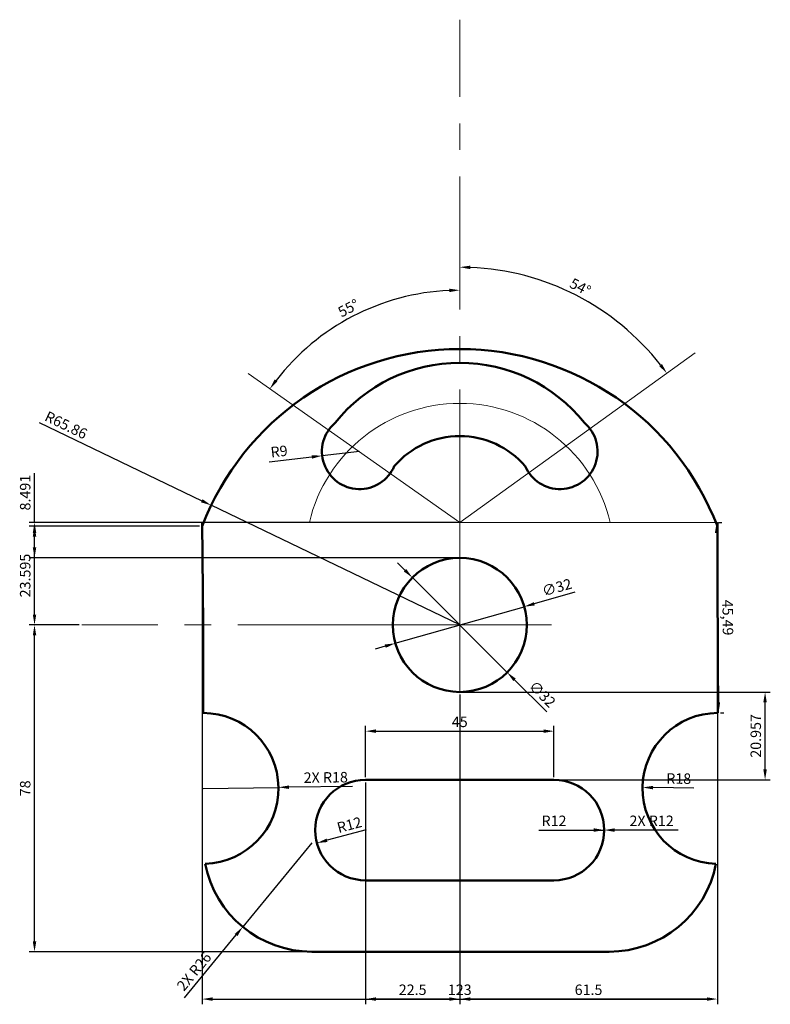
# Model space of a CAD drawing. Units: millimetres. Extents: x 3066 to 3245, y 1227 to 1462.
import ezdxf

# ---------------------------------------------------------------- set-up
doc = ezdxf.new("R2010")
doc.units = ezdxf.units.MM
doc.linetypes.add('CENTER', pattern=[50.8, 31.75, -6.35, 6.35, -6.35])
for name, color, linetype, lineweight in [('M-CNTR', 4, 'CENTER', 18), ('M-CONS', 8, 'Continuous', 13), ('M-DIMS', 2, 'Continuous', 25), ('M-OUTL', 7, 'Continuous', 50)]:
    doc.layers.add(name, color=color, linetype=linetype, lineweight=lineweight)
doc.styles.get("Standard").update_dxf_attribs({"font": 'arial.ttf'})
doc.dimstyles.new('ISO-25', dxfattribs={"dimtxt": 2.5, "dimasz": 2.5, "dimexe": 1.25, "dimexo": 0.625, "dimtad": 1, "dimtxsty": 'Standard', "dimcen": 2.5, "dimadec": 0, "dimazin": 0, "dimtfac": 1, "dimtmove": 0, "dimatfit": 3, "dimfxl": 1, "dimarcsym": 0})

# ---------------------------------------------------------------- blocks, each defined once
blk = doc.blocks.new('*D1')
at = {"layer": 'Defpoints', "color": 0, "transparency": 16777216}
for p in [(3193.22, 1291.89), (3148.22, 1280.28), (3193.22, 1280.28)]:
    blk.add_point(p, dxfattribs=at)
at = {"layer": 'M-DIMS', "color": 0, "lineweight": -2, "transparency": 16777216}
for p, q in [((3148.22, 1280.91), (3148.22, 1293.14)), ((3193.22, 1280.91), (3193.22, 1293.14)), ((3150.72, 1291.89), (3190.72, 1291.89))]:
    blk.add_line(p, q, dxfattribs=at)
at = {"layer": 'M-DIMS', "color": 0, "transparency": 16777216}
for points in [[(3150.72, 1292.31), (3150.72, 1291.48), (3148.22, 1291.89)], [(3190.72, 1292.31), (3190.72, 1291.48), (3193.22, 1291.89)]]:
    blk.add_solid(points, dxfattribs=at)
at = {"layer": 'M-DIMS', "color": 0, "transparency": 16777216, "insert": (3170.72, 1293.79), "char_height": 2.5, "attachment_point": 5}
blk.add_mtext('45', dxfattribs=at)
blk = doc.blocks.new('*D2')
at = {"layer": 'Defpoints', "color": 0, "transparency": 16777216}
for p in [(3186.11, 1321.61), (3155.33, 1312.86)]:
    blk.add_point(p, dxfattribs=at)
at = {"layer": 'M-DIMS', "color": 0, "lineweight": -2, "transparency": 16777216}
for p, q in [((3198.16, 1325.04), (3188.51, 1322.3)), ((3155.33, 1312.86), (3186.11, 1321.61)), ((3152.92, 1312.18), (3150.52, 1311.49))]:
    blk.add_line(p, q, dxfattribs=at)
at = {"layer": 'M-DIMS', "color": 0, "transparency": 16777216}
for points in [[(3188.4, 1322.7), (3188.63, 1321.9), (3186.11, 1321.61)], [(3152.81, 1312.58), (3153.04, 1311.78), (3155.33, 1312.86)]]:
    blk.add_solid(points, dxfattribs=at)
at = {"layer": 'M-DIMS', "color": 0, "transparency": 16777216, "insert": (3194, 1325.91), "char_height": 2.5, "attachment_point": 5, "rotation": 15.8749}
blk.add_mtext('∅32', dxfattribs=at)
blk = doc.blocks.new('*D3')
at = {"layer": 'Defpoints', "color": 0, "transparency": 16777216}
for p in [(3214.36, 1278.45), (3232.36, 1278.24)]:
    blk.add_point(p, dxfattribs=at)
at = {"layer": 'M-DIMS', "color": 0, "lineweight": -2, "transparency": 16777216}
blk.add_line((3226.58, 1278.31), (3216.86, 1278.42), dxfattribs=at)
at = {"layer": 'M-DIMS', "color": 0, "transparency": 16777216}
blk.add_solid([(3216.86, 1278.83), (3216.85, 1278), (3214.36, 1278.45)], dxfattribs=at)
at = {"layer": 'M-DIMS', "color": 0, "transparency": 16777216, "insert": (3222.99, 1280.25), "char_height": 2.5, "attachment_point": 5, "rotation": 359.3352}
blk.add_mtext('R18', dxfattribs=at)
blk = doc.blocks.new('*D4')
at = {"layer": 'Defpoints', "color": 0, "transparency": 16777216}
for p in [(3146.81, 1358.67), (3137.87, 1357.64)]:
    blk.add_point(p, dxfattribs=at)
at = {"layer": 'M-DIMS', "color": 0, "lineweight": -2, "transparency": 16777216}
for p, q in [((3146.81, 1358.67), (3137.87, 1357.64)), ((3125.21, 1356.17), (3135.39, 1357.35))]:
    blk.add_line(p, q, dxfattribs=at)
at = {"layer": 'M-DIMS', "color": 0, "transparency": 16777216}
blk.add_solid([(3135.34, 1357.76), (3135.44, 1356.94), (3137.87, 1357.64)], dxfattribs=at)
at = {"layer": 'M-DIMS', "color": 0, "transparency": 16777216, "insert": (3127.62, 1358.36), "char_height": 2.5, "attachment_point": 5, "rotation": 6.6057}
blk.add_mtext('R9', dxfattribs=at)
blk = doc.blocks.new('*D5')
at = {"layer": 'Defpoints', "color": 0, "transparency": 16777216}
for p in [(3148.22, 1268.28), (3136.62, 1265.19)]:
    blk.add_point(p, dxfattribs=at)
at = {"layer": 'M-DIMS', "color": 0, "lineweight": -2, "transparency": 16777216}
blk.add_line((3148.41, 1268.33), (3139.04, 1265.84), dxfattribs=at)
at = {"layer": 'M-DIMS', "color": 0, "transparency": 16777216}
blk.add_solid([(3138.93, 1266.24), (3139.15, 1265.43), (3136.62, 1265.19)], dxfattribs=at)
at = {"layer": 'M-DIMS', "color": 0, "transparency": 16777216, "insert": (3144.45, 1269.22), "char_height": 2.5, "attachment_point": 5, "rotation": 14.9155}
blk.add_mtext('R12', dxfattribs=at)
blk = doc.blocks.new('*D6')
at = {"layer": 'Defpoints', "color": 0, "transparency": 16777216}
for p in [(3193.22, 1268.28), (3205.22, 1268.28)]:
    blk.add_point(p, dxfattribs=at)
at = {"layer": 'M-DIMS', "color": 0, "lineweight": -2, "transparency": 16777216}
blk.add_line((3189.62, 1268.28), (3202.72, 1268.28), dxfattribs=at)
at = {"layer": 'M-DIMS', "color": 0, "transparency": 16777216}
blk.add_solid([(3202.72, 1268.7), (3202.72, 1267.86), (3205.22, 1268.28)], dxfattribs=at)
at = {"layer": 'M-DIMS', "color": 0, "transparency": 16777216, "insert": (3193.22, 1270.16), "char_height": 2.5, "attachment_point": 5}
blk.add_mtext('R12', dxfattribs=at)
blk = doc.blocks.new('*D7')
at = {"layer": 'Defpoints', "color": 0, "transparency": 16777216}
for p in [(3231.86, 1341.73), (3232.32, 1296.24), (3232.5, 1296.24)]:
    blk.add_point(p, dxfattribs=at)
at = {"layer": 'M-DIMS', "color": 0, "lineweight": -2, "transparency": 16777216}
for p, q in [((3232.48, 1341.74), (3233.29, 1341.74)), ((3232.06, 1339.23), (3232.47, 1298.74)), ((3232.94, 1296.24), (3233.75, 1296.25))]:
    blk.add_line(p, q, dxfattribs=at)
at = {"layer": 'M-DIMS', "color": 0, "transparency": 16777216}
for points in [[(3232.48, 1339.24), (3231.65, 1339.23), (3232.04, 1341.73)], [(3232.89, 1298.74), (3232.05, 1298.74), (3232.5, 1296.24)]]:
    blk.add_solid(points, dxfattribs=at)
at = {"layer": 'M-DIMS', "color": 0, "transparency": 16777216, "insert": (3234.4, 1319.01), "char_height": 2.5, "attachment_point": 5, "rotation": 270.5755}
blk.add_mtext('45,49', dxfattribs=at)
blk = doc.blocks.new('*D8')
at = {"layer": 'Defpoints', "color": 0, "transparency": 16777216}
for p in [(3170.72, 1461.73), (3153.32, 1394.36), (3120.17, 1377.27), (3170.72, 1341.73), (3170.72, 1341.73)]:
    blk.add_point(p, dxfattribs=at)
at = {"layer": 'M-DIMS', "color": 0, "lineweight": -2, "transparency": 16777216}
blk.add_arc((3170.72, 1341.73), 55.43, 92.5844, 142.3049, dxfattribs=at)
at = {"layer": 'M-DIMS', "color": 0, "transparency": 16777216}
for points in [[(3168.21, 1397.52), (3168.23, 1396.69), (3170.72, 1397.16)], [(3127.19, 1375.38), (3126.52, 1375.87), (3125.37, 1373.61)]]:
    blk.add_solid(points, dxfattribs=at)
at = {"layer": 'M-DIMS', "color": 0, "transparency": 16777216, "insert": (3144.3, 1392.6), "char_height": 2.5, "attachment_point": 5, "rotation": 27.4446}
blk.add_mtext('55°', dxfattribs=at)
blk = doc.blocks.new('*D9')
at = {"layer": 'Defpoints', "color": 0, "transparency": 16777216}
for p in [(3170.72, 1461.73), (3206.68, 1390.9), (3226.96, 1382.2), (3170.72, 1341.73), (3170.72, 1341.73)]:
    blk.add_point(p, dxfattribs=at)
at = {"layer": 'M-DIMS', "color": 0, "lineweight": -2, "transparency": 16777216}
blk.add_arc((3170.72, 1341.73), 60.92, 38.0865, 87.6486, dxfattribs=at)
at = {"layer": 'M-DIMS', "color": 0, "transparency": 16777216}
for points in [[(3173.21, 1402.18), (3173.23, 1403.02), (3170.72, 1402.65)], [(3219, 1379.56), (3218.34, 1379.06), (3220.17, 1377.31)]]:
    blk.add_solid(points, dxfattribs=at)
at = {"layer": 'M-DIMS', "color": 0, "transparency": 16777216, "insert": (3199.37, 1397.63), "char_height": 2.5, "attachment_point": 5, "rotation": 332.8675}
blk.add_mtext('54°', dxfattribs=at)
blk = doc.blocks.new('*D10')
at = {"layer": 'Defpoints', "color": 0, "transparency": 16777216}
for p in [(3109.22, 1341.73), (3232.22, 1341.73), (3232.22, 1227.94)]:
    blk.add_point(p, dxfattribs=at)
at = {"layer": 'M-DIMS', "color": 0, "lineweight": -2, "transparency": 16777216}
for p, q in [((3109.22, 1341.1), (3109.22, 1226.69)), ((3232.22, 1341.1), (3232.22, 1226.69)), ((3111.72, 1227.94), (3229.72, 1227.94))]:
    blk.add_line(p, q, dxfattribs=at)
at = {"layer": 'M-DIMS', "color": 0, "transparency": 16777216}
for points in [[(3111.72, 1228.35), (3111.72, 1227.52), (3109.22, 1227.94)], [(3229.72, 1228.35), (3229.72, 1227.52), (3232.22, 1227.94)]]:
    blk.add_solid(points, dxfattribs=at)
at = {"layer": 'M-DIMS', "color": 0, "transparency": 16777216, "insert": (3170.72, 1229.84), "char_height": 2.5, "attachment_point": 5}
blk.add_mtext('123', dxfattribs=at)
blk = doc.blocks.new('*D11')
at = {"layer": 'Defpoints', "color": 0, "transparency": 16777216}
for p in [(3069.19, 1317.24), (3080.49, 1317.24), (3135.44, 1239.24)]:
    blk.add_point(p, dxfattribs=at)
at = {"layer": 'M-DIMS', "color": 0, "lineweight": -2, "transparency": 16777216}
for p, q in [((3079.87, 1317.24), (3067.94, 1317.24)), ((3069.19, 1241.74), (3069.19, 1314.74)), ((3134.81, 1239.24), (3067.94, 1239.24))]:
    blk.add_line(p, q, dxfattribs=at)
at = {"layer": 'M-DIMS', "color": 0, "transparency": 16777216}
for points in [[(3068.78, 1314.74), (3069.61, 1314.74), (3069.19, 1317.24)], [(3068.78, 1241.74), (3069.61, 1241.74), (3069.19, 1239.24)]]:
    blk.add_solid(points, dxfattribs=at)
at = {"layer": 'M-DIMS', "color": 0, "transparency": 16777216, "insert": (3067.29, 1278.24), "char_height": 2.5, "attachment_point": 5, "rotation": 90}
blk.add_mtext('78', dxfattribs=at)
blk = doc.blocks.new('*D12')
at = {"layer": 'Defpoints', "color": 0, "transparency": 16777216}
for p in [(3170.72, 1301.24), (3243.62, 1301.24), (3193.22, 1280.28)]:
    blk.add_point(p, dxfattribs=at)
at = {"layer": 'M-DIMS', "color": 0, "lineweight": -2, "transparency": 16777216}
for p, q in [((3171.34, 1301.24), (3244.87, 1301.24)), ((3243.62, 1282.78), (3243.62, 1298.74)), ((3193.84, 1280.28), (3244.87, 1280.28))]:
    blk.add_line(p, q, dxfattribs=at)
at = {"layer": 'M-DIMS', "color": 0, "transparency": 16777216}
for points in [[(3243.2, 1298.74), (3244.03, 1298.74), (3243.62, 1301.24)], [(3243.2, 1282.78), (3244.03, 1282.78), (3243.62, 1280.28)]]:
    blk.add_solid(points, dxfattribs=at)
at = {"layer": 'M-DIMS', "color": 0, "transparency": 16777216, "insert": (3241.72, 1290.76), "char_height": 2.5, "attachment_point": 5, "rotation": 90}
blk.add_mtext('20.957', dxfattribs=at)
blk = doc.blocks.new('*D13')
at = {"layer": 'Defpoints', "color": 0, "transparency": 16777216}
for p in [(3069.19, 1341.73), (3170.72, 1341.73), (3170.72, 1333.24)]:
    blk.add_point(p, dxfattribs=at)
at = {"layer": 'M-DIMS', "color": 0, "lineweight": -2, "transparency": 16777216}
for p, q in [((3069.19, 1341.73), (3069.19, 1353.44)), ((3170.09, 1341.73), (3067.94, 1341.73)), ((3069.19, 1335.74), (3069.19, 1339.23)), ((3170.09, 1333.24), (3067.94, 1333.24))]:
    blk.add_line(p, q, dxfattribs=at)
at = {"layer": 'M-DIMS', "color": 0, "transparency": 16777216}
for points in [[(3068.78, 1339.23), (3069.61, 1339.23), (3069.19, 1341.73)], [(3068.78, 1335.74), (3069.61, 1335.74), (3069.19, 1333.24)]]:
    blk.add_solid(points, dxfattribs=at)
at = {"layer": 'M-DIMS', "color": 0, "transparency": 16777216, "insert": (3067.29, 1348.83), "char_height": 2.5, "attachment_point": 5, "rotation": 90}
blk.add_mtext('8.491', dxfattribs=at)
blk = doc.blocks.new('*D14')
at = {"layer": 'Defpoints', "color": 0, "transparency": 16777216}
for p in [(3232.22, 1341.73), (3170.72, 1301.24), (3170.72, 1227.94)]:
    blk.add_point(p, dxfattribs=at)
at = {"layer": 'M-DIMS', "color": 0, "lineweight": -2, "transparency": 16777216}
for p, q in [((3232.22, 1341.1), (3232.22, 1226.69)), ((3170.72, 1300.61), (3170.72, 1226.69)), ((3229.72, 1227.94), (3173.22, 1227.94))]:
    blk.add_line(p, q, dxfattribs=at)
at = {"layer": 'M-DIMS', "color": 0, "transparency": 16777216}
for points in [[(3173.22, 1228.35), (3173.22, 1227.52), (3170.72, 1227.94)], [(3229.72, 1228.35), (3229.72, 1227.52), (3232.22, 1227.94)]]:
    blk.add_solid(points, dxfattribs=at)
at = {"layer": 'M-DIMS', "color": 0, "transparency": 16777216, "insert": (3201.47, 1229.84), "char_height": 2.5, "attachment_point": 5}
blk.add_mtext('61.5', dxfattribs=at)
blk = doc.blocks.new('*D15')
at = {"layer": 'Defpoints', "color": 0, "transparency": 16777216}
for p in [(3170.72, 1301.24), (3148.22, 1280.28), (3148.22, 1227.94)]:
    blk.add_point(p, dxfattribs=at)
at = {"layer": 'M-DIMS', "color": 0, "lineweight": -2, "transparency": 16777216}
for p, q in [((3170.72, 1300.61), (3170.72, 1226.69)), ((3148.22, 1279.66), (3148.22, 1226.69)), ((3168.22, 1227.94), (3150.72, 1227.94))]:
    blk.add_line(p, q, dxfattribs=at)
at = {"layer": 'M-DIMS', "color": 0, "transparency": 16777216}
for points in [[(3150.72, 1228.35), (3150.72, 1227.52), (3148.22, 1227.94)], [(3168.22, 1228.35), (3168.22, 1227.52), (3170.72, 1227.94)]]:
    blk.add_solid(points, dxfattribs=at)
at = {"layer": 'M-DIMS', "color": 0, "transparency": 16777216, "insert": (3159.47, 1229.84), "char_height": 2.5, "attachment_point": 5}
blk.add_mtext('22.5', dxfattribs=at)
blk = doc.blocks.new('*D16')
at = {"layer": 'Defpoints', "color": 0, "transparency": 16777216}
for p in [(3069.19, 1340.83), (3109.23, 1340.83), (3080.49, 1317.24)]:
    blk.add_point(p, dxfattribs=at)
at = {"layer": 'M-DIMS', "color": 0, "lineweight": -2, "transparency": 16777216}
for p, q in [((3108.6, 1340.83), (3067.94, 1340.83)), ((3069.19, 1319.74), (3069.19, 1338.33)), ((3079.87, 1317.24), (3067.94, 1317.24))]:
    blk.add_line(p, q, dxfattribs=at)
at = {"layer": 'M-DIMS', "color": 0, "transparency": 16777216}
for points in [[(3068.78, 1338.33), (3069.61, 1338.33), (3069.19, 1340.83)], [(3068.78, 1319.74), (3069.61, 1319.74), (3069.19, 1317.24)]]:
    blk.add_solid(points, dxfattribs=at)
at = {"layer": 'M-DIMS', "color": 0, "transparency": 16777216, "insert": (3067.29, 1329.04), "char_height": 2.5, "attachment_point": 5, "rotation": 90}
blk.add_mtext('23.595', dxfattribs=at)
blk = doc.blocks.new('*D17')
at = {"layer": 'Defpoints', "color": 0, "transparency": 16777216}
for p in [(3111.37, 1345.81), (3170.72, 1317.24)]:
    blk.add_point(p, dxfattribs=at)
at = {"layer": 'M-DIMS', "color": 0, "lineweight": -2, "transparency": 16777216}
for p, q in [((3070.33, 1365.57), (3109.12, 1346.89)), ((3170.72, 1317.24), (3111.37, 1345.81))]:
    blk.add_line(p, q, dxfattribs=at)
at = {"layer": 'M-DIMS', "color": 0, "transparency": 16777216}
blk.add_solid([(3109.3, 1347.27), (3108.94, 1346.52), (3111.37, 1345.81)], dxfattribs=at)
at = {"layer": 'M-DIMS', "color": 0, "transparency": 16777216, "insert": (3076.59, 1364.66), "char_height": 2.5, "attachment_point": 5, "rotation": 334.293}
blk.add_mtext('R65.86', dxfattribs=at)
blk = doc.blocks.new('*D18')
at = {"layer": 'Defpoints', "color": 0, "transparency": 16777216}
for p in [(3159.41, 1328.55), (3182.03, 1305.92)]:
    blk.add_point(p, dxfattribs=at)
at = {"layer": 'M-DIMS', "color": 0, "lineweight": -2, "transparency": 16777216}
for p, q in [((3157.64, 1330.32), (3155.87, 1332.09)), ((3159.41, 1328.55), (3182.03, 1305.92)), ((3191.48, 1296.48), (3183.8, 1304.16))]:
    blk.add_line(p, q, dxfattribs=at)
at = {"layer": 'M-DIMS', "color": 0, "transparency": 16777216}
for points in [[(3157.93, 1330.61), (3157.34, 1330.03), (3159.41, 1328.55)], [(3184.09, 1304.45), (3183.51, 1303.86), (3182.03, 1305.92)]]:
    blk.add_solid(points, dxfattribs=at)
at = {"layer": 'M-DIMS', "color": 0, "transparency": 16777216, "insert": (3190.21, 1300.53), "char_height": 2.5, "attachment_point": 5, "rotation": 314.9993}
blk.add_mtext('∅32', dxfattribs=at)
blk = doc.blocks.new('*D19')
at = {"layer": 'Defpoints', "color": 0, "transparency": 16777216}
for p in [(3135.44, 1265.24), (3118.91, 1245.17)]:
    blk.add_point(p, dxfattribs=at)
at = {"layer": 'M-DIMS', "color": 0, "lineweight": -2, "transparency": 16777216}
for p, q in [((3135.44, 1265.24), (3118.91, 1245.17)), ((3104.98, 1228.24), (3117.32, 1243.24))]:
    blk.add_line(p, q, dxfattribs=at)
at = {"layer": 'M-DIMS', "color": 0, "transparency": 16777216}
blk.add_solid([(3117, 1243.5), (3117.65, 1242.97), (3118.91, 1245.17)], dxfattribs=at)
at = {"layer": 'M-DIMS', "color": 0, "transparency": 16777216, "insert": (3107.53, 1234.33), "char_height": 2.5, "attachment_point": 5, "rotation": 50.5361}
blk.add_mtext('2X R26', dxfattribs=at)
blk = doc.blocks.new('*D20')
at = {"layer": 'Defpoints', "color": 0, "transparency": 16777216}
for p in [(3193.22, 1268.28), (3205.22, 1268.28)]:
    blk.add_point(p, dxfattribs=at)
at = {"layer": 'M-DIMS', "color": 0, "lineweight": -2, "transparency": 16777216}
for p, q in [((3193.22, 1268.28), (3205.22, 1268.28)), ((3222.83, 1268.28), (3207.72, 1268.28))]:
    blk.add_line(p, q, dxfattribs=at)
at = {"layer": 'M-DIMS', "color": 0, "transparency": 16777216}
blk.add_solid([(3207.72, 1268.7), (3207.72, 1267.86), (3205.22, 1268.28)], dxfattribs=at)
at = {"layer": 'M-DIMS', "color": 0, "transparency": 16777216, "insert": (3216.53, 1270.16), "char_height": 2.5, "attachment_point": 5, "rotation": 359.9991}
blk.add_mtext('2X R12', dxfattribs=at)
blk = doc.blocks.new('*D21')
at = {"layer": 'Defpoints', "color": 0, "transparency": 16777216}
for p in [(3109.44, 1278.24), (3127.44, 1278.48)]:
    blk.add_point(p, dxfattribs=at)
at = {"layer": 'M-DIMS', "color": 0, "lineweight": -2, "transparency": 16777216}
for p, q in [((3145.08, 1278.72), (3129.94, 1278.51)), ((3109.44, 1278.24), (3127.44, 1278.48))]:
    blk.add_line(p, q, dxfattribs=at)
at = {"layer": 'M-DIMS', "color": 0, "transparency": 16777216}
blk.add_solid([(3129.93, 1278.93), (3129.94, 1278.1), (3127.44, 1278.48)], dxfattribs=at)
at = {"layer": 'M-DIMS', "color": 0, "transparency": 16777216, "insert": (3138.73, 1280.53), "char_height": 2.5, "attachment_point": 5, "rotation": 0.7694}
blk.add_mtext('2X R18', dxfattribs=at)

msp = doc.modelspace()

# ---------------------------------------------------------------- linework, layer by layer
at = {"layer": 'M-CNTR'}
for p, q in [((3170.719, 1341.7293), (3170.719, 1461.7293)), ((3170.719, 1341.7293), (3170.719, 1392.9044)), ((3170.719, 1333.2383), (3170.719, 1341.7293)), ((3170.719, 1318.2713), (3170.719, 1333.2383)), ((3170.719, 1333.2383), (3170.719, 1301.2383)), ((3149.4468, 1317.2383), (3080.4934, 1317.2383)), ((3170.719, 1317.2383), (3149.4468, 1317.2383)), ((3170.719, 1317.2383), (3192.5887, 1317.2383))]:
    msp.add_line(p, q, dxfattribs=at)
at = {"layer": 'M-CONS'}
for p, q in [((3170.719, 1341.7293), (3226.9647, 1382.1981)), ((3170.719, 1341.7293), (3120.1663, 1377.2724)), ((3109.219, 1341.7293), (3232.219, 1341.7293)), ((3232.219, 1341.7293), (3170.719, 1341.7293))]:
    msp.add_line(p, q, dxfattribs=at)
msp.add_arc((3170.719, 1333.2383), 36.9014, 13.302905, 166.697095, dxfattribs=at)
at = {"layer": 'M-OUTL'}
for p, q in [((3109.4391, 1317.2383), (3109.219, 1341.7293)), ((3232.3167, 1296.2383), (3232.219, 1341.7293)), ((3109.4391, 1317.2383), (3109.4391, 1309.4383)), ((3109.4391, 1317.2383), (3109.4391, 1296.2383)), ((3109.4391, 1309.4383), (3109.4391, 1304.0383)), ((3148.219, 1280.2812), (3193.219, 1280.2812)), ((3148.219, 1256.2812), (3193.219, 1256.2812)), ((3135.4391, 1239.2383), (3206.3832, 1239.2383))]:
    msp.add_line(p, q, dxfattribs=at)
msp.add_circle((3170.719, 1317.2383), 16, dxfattribs=at)
for centre, radius, start, end in [((3170.719, 1317.2383), 65.8635, 20.968169, 159.007467), ((3170.719, 1341.7293), 38.0899, 38.656088, 141.343912), ((3146.8128, 1358.6727), 9, 130.446106, 336.96821), ((3194.6251, 1358.6727), 9, 203.03179, 49.553894), ((3170.719, 1341.7293), 20.5974, 40.666093, 139.333907), ((3109.4391, 1278.2383), 18, 271.540881, 90), ((3232.3553, 1278.2383), 18, 90.123036, 268.547367), ((3148.219, 1268.2812), 12, 90, 270), ((3193.219, 1268.2812), 12, 270, 90), ((3135.4391, 1265.2383), 26, 191.072873, 270), ((3206.3832, 1265.2383), 26, 270, 348.925501)]:
    msp.add_arc(centre, radius, start, end, dxfattribs=at)

# ---------------------------------------------------------------- dimensions: what is measured, and where the dimension line sits
at = {"layer": 'M-DIMS'}
for base, line1, line2, picture, middle in [((3153.3176, 1394.3571), ((3170.719, 1341.7293), (3170.719, 1461.7293)), ((3170.719, 1341.7293), (3120.1663, 1377.2724)), '*D8', (3144.2977, 1392.604)), ((3206.6792, 1390.9048), ((3170.719, 1341.7293), (3226.9647, 1382.1981)), ((3170.719, 1341.7293), (3170.719, 1461.7293)), '*D9', (3199.3668, 1397.6338))]:
    dim = msp.add_angular_dim_2l(base=base, line1=line1, line2=line2, dimstyle='ISO-25', override={"dimclrd": 0, "dimclre": 0, "dimclrt": 0}, dxfattribs=at)
    dim.commit()
    dim.dimension.update_dxf_attribs({"geometry": picture, "text_midpoint": middle})
for center, mpoint, override, picture, middle in [((3170.719, 1317.2383), (3111.3744, 1345.8079), {"dimdec": 2, "dimlfac": 1, "dimrnd": 0, "dimzin": 0, "dimdsep": 46, "dimlunit": 2}, '*D17', (3075.7677, 1362.9496)), ((3146.8128, 1358.6727), (3137.8726, 1357.6374), {"dimclrd": 0, "dimclre": 0, "dimclrt": 0}, '*D4', (3127.8339, 1356.4749)), ((3232.3553, 1278.2383), (3214.3565, 1278.4471), {"dimclrd": 0, "dimclre": 0, "dimclrt": 0}, '*D3', (3222.9704, 1278.3472)), ((3148.219, 1268.2812), (3136.6233, 1265.1925), {"dimclrd": 0, "dimclre": 0, "dimclrt": 0}, '*D5', (3144.9327, 1267.4058)), ((3193.219, 1268.2812), (3205.219, 1268.2812), {"dimclrd": 0, "dimclre": 0, "dimclrt": 0}, '*D6', (3193.219, 1268.2812))]:
    dim = msp.add_radius_dim(center=center, mpoint=mpoint, dimstyle='ISO-25', override=override, dxfattribs=at)
    dim.commit()
    dim.dimension.update_dxf_attribs({"geometry": picture, "text_midpoint": middle, "dimtype": 164})
for base, p1, p2, override, picture, middle in [((3069.1934, 1341.7293), (3170.719, 1333.2383), (3170.719, 1341.7293), {"dimdec": 3, "dimlfac": 1, "dimrnd": 0, "dimzin": 0, "dimdsep": 46, "dimlunit": 2}, '*D13', (3067.292, 1348.8328)), ((3069.1934, 1340.8336), (3080.4934, 1317.2383), (3109.227, 1340.8336), {"dimdec": 3, "dimlfac": 1, "dimrnd": 0, "dimzin": 0, "dimdsep": 46, "dimlunit": 2}, '*D16', (3067.2911, 1329.036)), ((3069.1934, 1317.2383), (3135.4391, 1239.2383), (3080.4934, 1317.2383), {"dimdec": 0, "dimlfac": 1, "dimrnd": 0, "dimzin": 0, "dimdsep": 46, "dimlunit": 2}, '*D11', (3067.292, 1278.2383)), ((3243.6167, 1301.2383), (3193.219, 1280.2812), (3170.719, 1301.2383), {"dimdec": 3, "dimlfac": 1, "dimrnd": 0, "dimzin": 0, "dimdsep": 46, "dimlunit": 2}, '*D12', (3241.7152, 1290.7597))]:
    dim = msp.add_linear_dim(base=base, p1=p1, p2=p2, angle=90, dimstyle='ISO-25', override=override, dxfattribs=at)
    dim.commit()
    dim.dimension.update_dxf_attribs({"geometry": picture, "text_midpoint": middle})
for base, p1, p2, override, picture, middle in [((3232.219, 1227.9383), (3109.219, 1341.7293), (3232.219, 1341.7293), {"dimdec": 0, "dimlfac": 1, "dimrnd": 0, "dimzin": 0, "dimdsep": 46, "dimlunit": 2}, '*D10', (3170.719, 1229.8406)), ((3170.719, 1227.9383), (3232.219, 1341.7293), (3170.719, 1301.2383), {"dimdec": 1, "dimlfac": 1, "dimrnd": 0, "dimzin": 0, "dimdsep": 46, "dimlunit": 2}, '*D14', (3201.469, 1229.8397)), ((3148.219, 1227.9383), (3170.719, 1301.2383), (3148.219, 1280.2812), {"dimdec": 1, "dimlfac": 1, "dimrnd": 0, "dimzin": 0, "dimdsep": 46, "dimlunit": 2}, '*D15', (3159.469, 1229.8397)), ((3193.219, 1291.8931), (3148.219, 1280.2812), (3193.219, 1280.2812), {"dimclrd": 0, "dimclre": 0, "dimclrt": 0}, '*D1', (3170.719, 1293.7895))]:
    dim = msp.add_linear_dim(base=base, p1=p1, p2=p2, dimstyle='ISO-25', override=override, dxfattribs=at)
    dim.commit()
    dim.dimension.update_dxf_attribs({"geometry": picture, "text_midpoint": middle})
dim = msp.add_aligned_dim(p1=(3231.8597, 1341.7293), p2=(3232.3167, 1296.2383), distance=0.1796, dimstyle='ISO-25', override={"dimclrd": 0, "dimclre": 0, "dimclrt": 0}, dxfattribs=at)
dim.commit()
dim.dimension.update_dxf_attribs({"geometry": '*D7', "text_midpoint": (3234.3951, 1319.0069)})
dim = msp.add_diameter_dim_2p(p1=(3159.4054, 1328.5521), p2=(3182.0326, 1305.9244), dimstyle='ISO-25', override={"dimdec": 0, "dimlfac": 1, "dimrnd": 0, "dimzin": 0, "dimdsep": 46, "dimlunit": 2}, dxfattribs=at)
dim.commit()
dim.dimension.update_dxf_attribs({"geometry": '*D18', "text_midpoint": (3188.8207, 1299.1361), "dimtype": 163})
dim = msp.add_diameter_dim_2p(p1=(3155.3292, 1312.8617), p2=(3186.1088, 1321.6149), dimstyle='ISO-25', override={"dimclrd": 0, "dimclre": 0, "dimclrt": 0}, dxfattribs=at)
dim.commit()
dim.dimension.update_dxf_attribs({"geometry": '*D2', "text_midpoint": (3193.9981, 1325.908)})
for center, mpoint, picture, middle in [((3109.4391, 1278.2383), (3127.4374, 1278.48), '*D21', (3138.7325, 1280.5333)), ((3193.219, 1268.2812), (3205.219, 1268.281), '*D20', (3216.5253, 1270.1618))]:
    dim = msp.add_radius_dim(center=center, mpoint=mpoint, text='2X <>', dimstyle='ISO-25', override={"dimdec": 0, "dimlfac": 1, "dimrnd": 0, "dimzin": 0, "dimdsep": 46, "dimlunit": 2}, dxfattribs=at)
    dim.commit()
    dim.dimension.update_dxf_attribs({"geometry": picture, "text_midpoint": middle})
dim = msp.add_radius_dim(center=(3135.4391, 1265.2383), mpoint=(3118.9137, 1245.1656), text='2X <>', dimstyle='ISO-25', override={"dimdec": 0, "dimlfac": 1, "dimrnd": 0, "dimzin": 0, "dimdsep": 46, "dimlunit": 2}, dxfattribs=at)
dim.commit()
dim.dimension.update_dxf_attribs({"geometry": '*D19', "text_midpoint": (3108.9985, 1233.122), "dimtype": 164})

doc.saveas('drawing.dxf')
